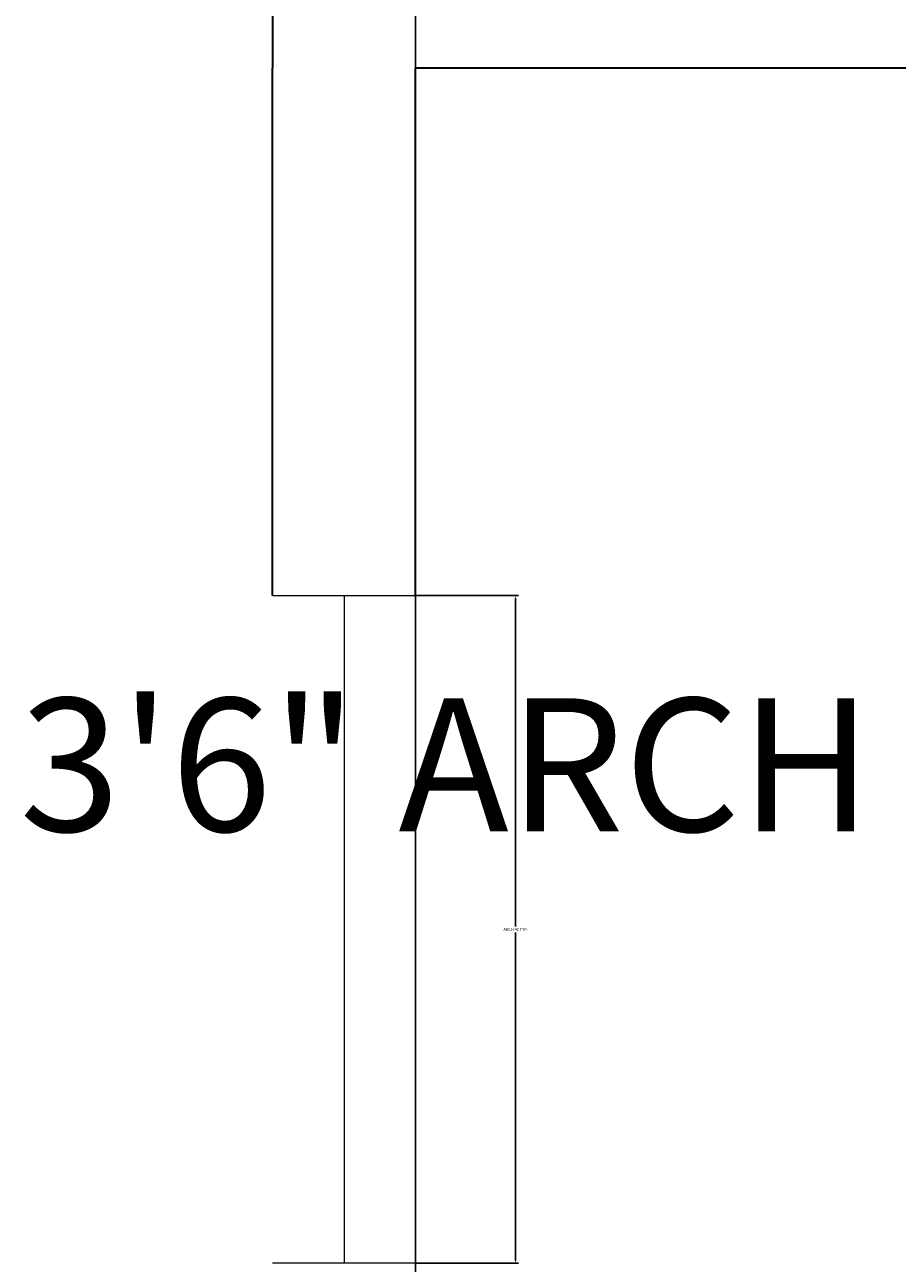
# Model space of a CAD drawing. Units: feet. Extents: x 1654 to 2985, y 1348 to 2230.
# Tile 34 of 53: x 2045 to 2100, y 1811 to 1889. Entities that reach past the tile are written whole.
import ezdxf

# ---------------------------------------------------------------- set-up
doc = ezdxf.new("R2010")
doc.units = ezdxf.units.FT
for name, color, linetype, lineweight in [('A-ANNO-DIMS', 2, 'Continuous', 18), ('A-ANNO-TEXT', 7, 'Continuous', 18), ('A-WALL', 7, 'Continuous', 35), ('A-WALL-OPEN', 4, 'Continuous', 18)]:
    doc.layers.add(name, color=color, linetype=linetype, lineweight=lineweight)
doc.styles.get("Standard").update_dxf_attribs({"font": 'arial.ttf'})
doc.dimstyles.get("Standard").update_dxf_attribs({"dimtxt": 0.18, "dimasz": 0.18, "dimexe": 0.18, "dimexo": 0.0625, "dimgap": 0.09, "dimtad": 0, "dimtih": 1, "dimtoh": 1, "dimdec": 4, "dimzin": 0, "dimdsep": 46, "dimtxsty": 'Standard', "dimcen": 0.09, "dimadec": 0, "dimazin": 0, "dimtfac": 1, "dimtdec": 4, "dimtofl": 0, "dimtmove": 0, "dimatfit": 3, "dimfxl": 1, "dimtolj": 1, "dimtzin": 0, "dimarcsym": 0})

# ---------------------------------------------------------------- blocks, each defined once
blk = doc.blocks.new('OPENING-LIVING-ARCH')
for p, q in [((0, 42), (9, 42)), ((4.5, 42), (4.5, 0)), ((9, 0), (0, 0))]:
    blk.add_line(p, q)
blk = doc.blocks.new('*D70')
at = {"layer": 'A-ANNO-DIMS', "color": 0, "lineweight": -2, "transparency": 16777216}
for p, q in [((2070.155, 1853.081), (2076.572, 1853.081)), ((2076.392, 1852.901), (2076.392, 1832.265)), ((2076.392, 1811.261), (2076.392, 1831.898)), ((2070.155, 1811.081), (2076.572, 1811.081))]:
    blk.add_line(p, q, dxfattribs=at)
at = {"layer": 'A-ANNO-DIMS', "color": 0, "transparency": 16777216}
for points in [[(2076.362, 1852.901), (2076.422, 1852.901), (2076.392, 1853.081)], [(2076.362, 1811.261), (2076.422, 1811.261), (2076.392, 1811.081)]]:
    blk.add_solid(points, dxfattribs=at)
at = {"layer": 'Defpoints', "color": 0, "transparency": 16777216}
for p in [(2070.092, 1853.081), (2076.392, 1853.081), (2070.092, 1811.081)]:
    blk.add_point(p, dxfattribs=at)
at = {"layer": 'A-ANNO-DIMS', "color": 0, "transparency": 16777216, "insert": (2076.392, 1832.081), "char_height": 0.18, "attachment_point": 5}
blk.add_mtext('\\A1;ARCH 42 TYP.', dxfattribs=at)
blk = doc.blocks.new('*D80')
at = {"layer": 'A-ANNO-DIMS', "color": 0, "lineweight": -2, "transparency": 16777216}
for p, q in [((2070.092, 2039.192), (2070.092, 1534.075)), ((2202.092, 2039.192), (2202.092, 1534.075)), ((2070.272, 1534.255), (2135.813, 1534.255)), ((2201.912, 1534.255), (2136.372, 1534.255))]:
    blk.add_line(p, q, dxfattribs=at)
at = {"layer": 'A-ANNO-DIMS', "color": 0, "transparency": 16777216}
for points in [[(2070.272, 1534.285), (2070.272, 1534.225), (2070.092, 1534.255)], [(2201.912, 1534.285), (2201.912, 1534.225), (2202.092, 1534.255)]]:
    blk.add_solid(points, dxfattribs=at)
at = {"layer": 'Defpoints', "color": 0, "transparency": 16777216}
for p in [(2070.092, 2039.255), (2202.092, 2039.255), (2202.092, 1534.255)]:
    blk.add_point(p, dxfattribs=at)
at = {"layer": 'A-ANNO-DIMS', "color": 0, "transparency": 16777216, "insert": (2136.092, 1534.255), "char_height": 0.18, "attachment_point": 5}
blk.add_mtext('\\A1;132', dxfattribs=at)

msp = doc.modelspace()

# ---------------------------------------------------------------- linework, layer by layer
at = {"layer": 'A-WALL'}
for p, q in [((2061.0924, 1895.2549), (2061.0924, 1886.2549)), ((2061.0924, 1853.0815), (2061.0924, 1886.2549)), ((2202.0924, 1886.2549), (2070.0924, 1886.2549)), ((2070.0924, 1853.0815), (2070.0924, 1886.2549))]:
    msp.add_line(p, q, dxfattribs=at)

# ---------------------------------------------------------------- block references
at = {"layer": 'A-WALL-OPEN'}
msp.add_blockref('OPENING-LIVING-ARCH', (2061.092, 1811.081), dxfattribs=at)

# ---------------------------------------------------------------- texts
at = {"layer": 'A-ANNO-TEXT'}
msp.add_text('3\'6" ARCH', height=8.38114, dxfattribs=at).set_placement((2045.1594, 1838.2451))

# ---------------------------------------------------------------- dimensions: what is measured, and where the dimension line sits
at = {"layer": 'A-ANNO-DIMS'}
dim = msp.add_linear_dim(base=(2202.0924, 1534.2549), p1=(2070.0924, 2039.2549), p2=(2202.0924, 2039.2549), dimstyle='Standard', override={"dimdec": 0, "dimlfac": 1, "dimrnd": 0, "dimzin": 0, "dimdsep": 46, "dimlunit": 2}, dxfattribs=at)
dim.commit()
dim.dimension.update_dxf_attribs({"geometry": '*D80', "text_midpoint": (2136.0924, 1534.2549)})
dim = msp.add_linear_dim(base=(2076.3924, 1853.0815), p1=(2070.0924, 1811.0815), p2=(2070.0924, 1853.0815), angle=90, text='ARCH <> TYP.', dimstyle='Standard', override={"dimdec": 0, "dimlfac": 1, "dimrnd": 0, "dimzin": 0, "dimdsep": 46, "dimlunit": 2}, dxfattribs=at)
dim.commit()
dim.dimension.update_dxf_attribs({"geometry": '*D70', "text_midpoint": (2076.3924, 1832.0815)})

doc.saveas('drawing.dxf')
